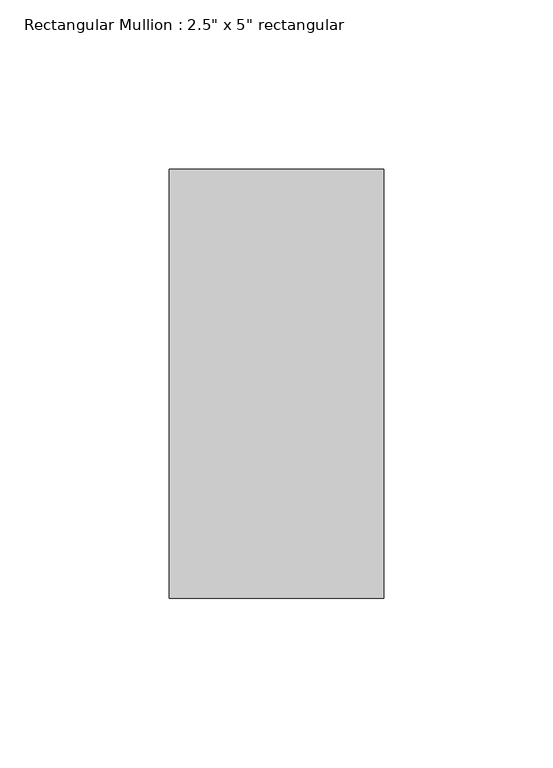
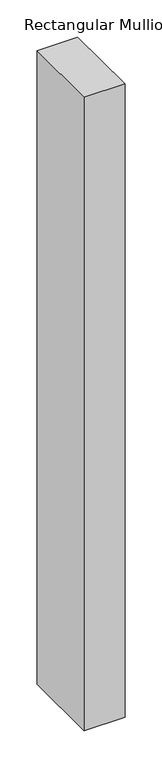
"""IFC4 building model written with IfcOpenShell, lengths in millimetres: member geometry."""

from ifc_helpers import new_model, si_unit, frame, origin, place, context, project, spatial, polyline, outline, extrude, source, transform, mapped, element, save


def member_c5c38a7a(model_context):
    return source(origin(), model_context, "Body", "SweptSolid", [
        extrude(outline(polyline([(31.75, 63.5), (31.75, -63.5), (-31.75, -63.5), (-31.75, 63.5), (31.75, 63.5)])), frame((0.0, 0.0, -1041.4), z_axis=(0.0, 0.0, 1.0), x_axis=(1.0, 0.0, 0.0)), (0.0, 0.0, 1.0), 1041.4),
    ])


if __name__ == "__main__":
    model = new_model("IFC4")
    model_context = context("Model", 3, world=origin())
    ifc_project = project(units=[si_unit("LENGTHUNIT", "METRE", prefix="MILLI")], contexts=[model_context])
    site = spatial("IfcSite", under=ifc_project)
    building = spatial("IfcBuilding", under=site)
    placement = place(None, origin())
    member_shape = member_c5c38a7a(model_context)
    element("IfcMember", 1, ObjectType="Rectangular Mullion : 2.5\" x 5\" rectangular", at=placement, inside=building, context=model_context, shape_type="MappedRepresentation", body=[
        mapped(member_shape, transform((0.0, 0.0, 0.0), x_axis=(1.0, 0.0, 0.0), y_axis=(0.0, 1.0, 0.0), z_axis=(0.0, 0.0, 1.0))),
    ])
    save(model, "model.ifc")

# Revit data of these elements
# Type "Rectangular Mullion : 2.5\" x 5\" rectangular"
#   built-in parameter 1007304 = 0.416667 (stored number, unit not read)
#   built-in parameter 1007301 = 0.104167 (stored number, unit not read)
#   built-in parameter 1007300 = 0.104167 (stored number, unit not read)
# Element 1 (IfcMember, "Rectangular Mullion : 2.5\" x 5\" rectangular")
#   Materials on its faces: "Aluminum"
# Materials
#   "Aluminum": class "Metal", colour RGB 247 247 247, transparency 0, Description = "Aluminum 6061", Cost = 0
